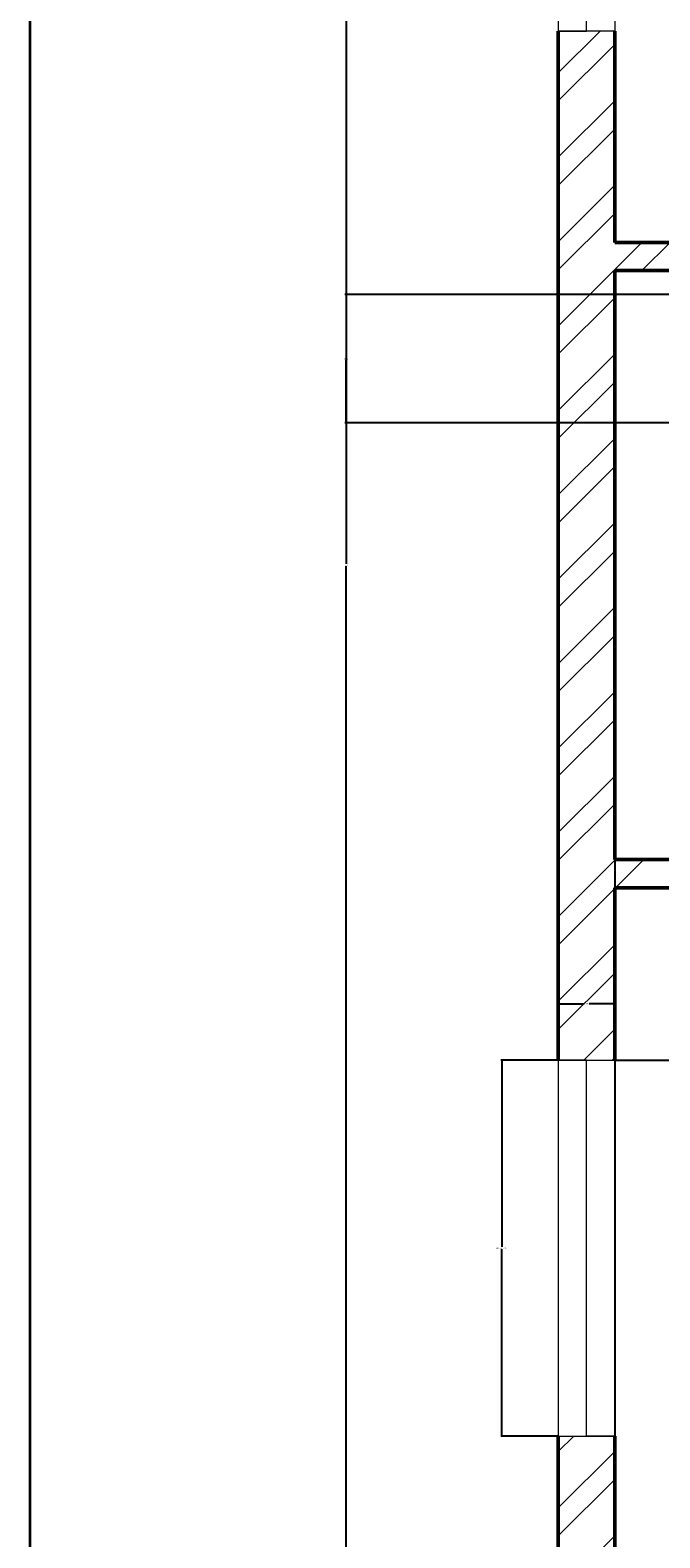
# Model space of a CAD drawing. Units: inches. Extents: x 2310 to 2937, y 1113 to 2410.
# Tile 3 of 23: x 2310 to 2411, y 1891 to 2132. Entities that reach past the tile are written whole.
import ezdxf

# ---------------------------------------------------------------- set-up
doc = ezdxf.new("R2010")
doc.units = ezdxf.units.IN
for name, color, linetype, lineweight in [('A-ANNO-DIMS', 2, 'Continuous', 18), ('A-ANNO-TTLB', 7, 'Continuous', 35), ('A-GLAZ', 191, 'Continuous', 20), ('A-WALL', 7, 'Continuous', 50), ('A-WALL-PATT', 85, 'Continuous', 13)]:
    doc.layers.add(name, color=color, linetype=linetype, lineweight=lineweight)
doc.styles.get("Standard").update_dxf_attribs({"font": 'arial.ttf'})
doc.dimstyles.get("Standard").update_dxf_attribs({"dimtxt": 0.18, "dimasz": 0.18, "dimexe": 0.18, "dimexo": 0.0625, "dimgap": 0.09, "dimtad": 0, "dimtih": 1, "dimtoh": 1, "dimdec": 4, "dimzin": 0, "dimdsep": 46, "dimtxsty": 'Standard', "dimcen": 0.09, "dimadec": 0, "dimazin": 0, "dimtfac": 1, "dimtdec": 4, "dimtofl": 0, "dimtmove": 0, "dimatfit": 3, "dimfxl": 1, "dimtolj": 1, "dimtzin": 0, "dimarcsym": 0})

# ---------------------------------------------------------------- blocks, each defined once
blk = doc.blocks.new('WIN-60IN')
for p, q in [((4.5, 60), (0, 60)), ((0, 60), (9, 60)), ((0, 60), (0, 0)), ((4.5, 0), (4.5, 60)), ((9, 60), (9, 0)), ((0, 0), (9, 0)), ((9, 0), (4.5, 0))]:
    blk.add_line(p, q)
blk = doc.blocks.new('*D27')
at = {"layer": 'A-ANNO-DIMS', "color": 0, "lineweight": -2, "transparency": 16777216}
for p, q in [((2394.42, 1967.52), (2385.31, 1967.52)), ((2385.49, 1967.34), (2385.49, 1937.71)), ((2385.49, 1907.7), (2385.49, 1937.34)), ((2394.42, 1907.52), (2385.31, 1907.52))]:
    blk.add_line(p, q, dxfattribs=at)
at = {"layer": 'A-ANNO-DIMS', "color": 0, "transparency": 16777216}
for points in [[(2385.46, 1967.34), (2385.52, 1967.34), (2385.49, 1967.52)], [(2385.46, 1907.7), (2385.52, 1907.7), (2385.49, 1907.52)]]:
    blk.add_solid(points, dxfattribs=at)
at = {"layer": 'Defpoints', "color": 0, "transparency": 16777216}
for p in [(2385.49, 1967.52), (2394.49, 1967.52), (2394.49, 1907.52)]:
    blk.add_point(p, dxfattribs=at)
at = {"layer": 'A-ANNO-DIMS', "color": 0, "transparency": 16777216, "insert": (2385.49, 1937.52), "char_height": 0.18, "attachment_point": 5}
blk.add_mtext('\\A1;WINDOW 60 TYP.', dxfattribs=at)
blk = doc.blocks.new('*D28')
at = {"layer": 'A-ANNO-DIMS', "color": 0, "lineweight": -2, "transparency": 16777216}
for p, q in [((2394.49, 1967.58), (2394.49, 1976.7)), ((2394.67, 1976.52), (2398.53, 1976.52)), ((2403.31, 1976.52), (2399.44, 1976.52)), ((2403.49, 1967.58), (2403.49, 1976.7))]:
    blk.add_line(p, q, dxfattribs=at)
at = {"layer": 'A-ANNO-DIMS', "color": 0, "transparency": 16777216}
for points in [[(2394.67, 1976.55), (2394.67, 1976.49), (2394.49, 1976.52)], [(2403.31, 1976.55), (2403.31, 1976.49), (2403.49, 1976.52)]]:
    blk.add_solid(points, dxfattribs=at)
at = {"layer": 'Defpoints', "color": 0, "transparency": 16777216}
for p in [(2403.49, 1976.52), (2394.49, 1967.52), (2403.49, 1967.52)]:
    blk.add_point(p, dxfattribs=at)
at = {"layer": 'A-ANNO-DIMS', "color": 0, "transparency": 16777216, "insert": (2398.99, 1976.52), "char_height": 0.18, "attachment_point": 5}
blk.add_mtext('\\A1;9 TYP.', dxfattribs=at)
blk = doc.blocks.new('*D40')
at = {"layer": 'A-ANNO-DIMS', "color": 0, "lineweight": -2, "transparency": 16777216}
for p, q in [((2394.42, 2356.51), (2360.46, 2356.51)), ((2360.64, 2356.33), (2360.64, 2046.7)), ((2360.64, 1736.69), (2360.64, 2046.33)), ((2394.42, 1736.51), (2360.46, 1736.51))]:
    blk.add_line(p, q, dxfattribs=at)
at = {"layer": 'A-ANNO-DIMS', "color": 0, "transparency": 16777216}
for points in [[(2360.61, 2356.33), (2360.67, 2356.33), (2360.64, 2356.51)], [(2360.61, 1736.69), (2360.67, 1736.69), (2360.64, 1736.51)]]:
    blk.add_solid(points, dxfattribs=at)
at = {"layer": 'Defpoints', "color": 0, "transparency": 16777216}
for p in [(2360.64, 2356.51), (2394.49, 2356.51), (2394.49, 1736.51)]:
    blk.add_point(p, dxfattribs=at)
at = {"layer": 'A-ANNO-DIMS', "color": 0, "transparency": 16777216, "insert": (2360.64, 2046.51), "char_height": 0.18, "attachment_point": 5}
blk.add_mtext('\\A1;620', dxfattribs=at)
blk = doc.blocks.new('*D57')
at = {"layer": 'A-ANNO-DIMS', "color": 0, "lineweight": -2, "transparency": 16777216}
for p, q in [((2403.55, 1995.01), (2858.02, 1995.01)), ((2857.84, 1994.83), (2857.84, 1981.45)), ((2857.84, 1967.7), (2857.84, 1981.09)), ((2403.55, 1967.52), (2858.02, 1967.52))]:
    blk.add_line(p, q, dxfattribs=at)
at = {"layer": 'A-ANNO-DIMS', "color": 0, "transparency": 16777216}
for points in [[(2857.81, 1994.83), (2857.87, 1994.83), (2857.84, 1995.01)], [(2857.81, 1967.7), (2857.87, 1967.7), (2857.84, 1967.52)]]:
    blk.add_solid(points, dxfattribs=at)
at = {"layer": 'Defpoints', "color": 0, "transparency": 16777216}
for p in [(2403.49, 1995.01), (2403.49, 1967.52), (2857.84, 1967.52)]:
    blk.add_point(p, dxfattribs=at)
at = {"layer": 'A-ANNO-DIMS', "color": 0, "transparency": 16777216, "insert": (2857.84, 1981.27), "char_height": 0.18, "attachment_point": 5}
blk.add_mtext('\\A1;27.49', dxfattribs=at)
blk = doc.blocks.new('*D65')
at = {"layer": 'A-ANNO-DIMS', "color": 0, "lineweight": -2, "transparency": 16777216}
for p, q in [((2403.49, 2093.45), (2403.49, 1649.5)), ((2436.46, 2093.45), (2436.46, 1649.5)), ((2403.67, 1649.68), (2419.58, 1649.68)), ((2436.28, 1649.68), (2420.37, 1649.68))]:
    blk.add_line(p, q, dxfattribs=at)
at = {"layer": 'A-ANNO-DIMS', "color": 0, "transparency": 16777216}
for points in [[(2403.67, 1649.71), (2403.67, 1649.65), (2403.49, 1649.68)], [(2436.28, 1649.71), (2436.28, 1649.65), (2436.46, 1649.68)]]:
    blk.add_solid(points, dxfattribs=at)
at = {"layer": 'Defpoints', "color": 0, "transparency": 16777216}
for p in [(2403.49, 2093.51), (2436.46, 2093.51), (2436.46, 1649.68)]:
    blk.add_point(p, dxfattribs=at)
at = {"layer": 'A-ANNO-DIMS', "color": 0, "transparency": 16777216, "insert": (2419.98, 1649.68), "char_height": 0.18, "attachment_point": 5}
blk.add_mtext('\\A1;32.98', dxfattribs=at)
blk = doc.blocks.new('*D67')
at = {"layer": 'A-ANNO-DIMS', "color": 0, "lineweight": -2, "transparency": 16777216}
for p, q in [((2684.42, 2089.69), (2360.46, 2089.69)), ((2360.64, 2089.51), (2360.64, 2079.64)), ((2360.64, 2069.41), (2360.64, 2079.28)), ((2684.42, 2069.23), (2360.46, 2069.23))]:
    blk.add_line(p, q, dxfattribs=at)
at = {"layer": 'A-ANNO-DIMS', "color": 0, "transparency": 16777216}
for points in [[(2360.61, 2089.51), (2360.67, 2089.51), (2360.64, 2089.69)], [(2360.61, 2069.41), (2360.67, 2069.41), (2360.64, 2069.23)]]:
    blk.add_solid(points, dxfattribs=at)
at = {"layer": 'Defpoints', "color": 0, "transparency": 16777216}
for p in [(2360.64, 2089.69), (2684.49, 2089.69), (2684.49, 2069.23)]:
    blk.add_point(p, dxfattribs=at)
at = {"layer": 'A-ANNO-DIMS', "color": 0, "transparency": 16777216, "insert": (2360.64, 2079.46), "char_height": 0.18, "attachment_point": 5}
blk.add_mtext('\\A1;20.46', dxfattribs=at)

msp = doc.modelspace()

# ---------------------------------------------------------------- hatches: boundary and pattern name
at = {"layer": 'A-WALL-PATT'}
h = msp.add_hatch(dxfattribs=at)
h.set_pattern_fill('ANSI32', color=256)
h.paths.add_polyline_path([(2639.1394, 2356.5139), (2563.662, 2356.5139), (2563.662, 2347.5139), (2606.9859, 2347.5139), (2606.9859, 2210.5139), (2514.2692, 2210.5139), (2514.2692, 2206.0139), (2606.9859, 2206.0139), (2606.9859, 2098.0139), (2602.689, 2098.0139), (2602.689, 2093.5139), (2615.5262, 2093.5139), (2615.5262, 2095.7639), (2615.5262, 2098.0139), (2611.4859, 2098.0139), (2611.4859, 2206.0139), (2703.9391, 2206.0139), (2703.9391, 2208.2639), (2703.9391, 2210.5139), (2611.4859, 2210.5139), (2611.4859, 2347.5139), (2639.1394, 2347.5139)])
h.paths.add_polyline_path([(2823.9859, 2356.5139), (2699.1394, 2356.5139), (2699.1394, 2347.5139), (2738.4859, 2347.5139), (2738.4859, 2343.9266), (2742.9859, 2343.9266), (2742.9859, 2347.5139), (2814.9859, 2347.5139), (2814.9859, 2336.76), (2823.9859, 2336.76)])
h.paths.add_polyline_path([(2823.9859, 2312.76), (2814.9859, 2312.76), (2814.9859, 2299.5139), (2742.9859, 2299.5139), (2742.9859, 2323.0159), (2740.7359, 2323.0159), (2738.4859, 2323.0159), (2738.4859, 2210.5139), (2734.5483, 2210.5139), (2734.5483, 2206.0139), (2746.8769, 2206.0139), (2746.8769, 2208.2639), (2746.8769, 2210.5139), (2742.9859, 2210.5139), (2742.9859, 2295.0139), (2814.9859, 2295.0139), (2814.9859, 2269.8977), (2823.9859, 2269.8977)])
h.paths.add_polyline_path([(2823.9859, 2210.5139), (2823.9859, 2233.8977), (2819.4859, 2233.8977), (2814.9859, 2233.8977), (2814.9859, 2210.5139), (2769.9745, 2210.5139), (2769.9745, 2206.0139), (2814.9859, 2206.0139), (2814.9859, 2178.3027), (2823.9859, 2178.3027)])
h.paths.add_polyline_path([(2823.9859, 2118.3027), (2819.4859, 2118.3027), (2814.9859, 2118.3027), (2814.9859, 2098.0139), (2647.0333, 2098.0139), (2647.0333, 2093.5139), (2814.9859, 2093.5139), (2814.9859, 1999.5139), (2650.6052, 1999.5139), (2650.6052, 1995.0139), (2814.9859, 1995.0139), (2814.9859, 1969.9784), (2823.9859, 1969.9784)])
h.paths.add_polyline_path([(2403.4859, 2093.5139), (2569.9888, 2093.5139), (2569.9888, 2095.7639), (2569.9888, 2098.0139), (2403.4859, 2098.0139), (2403.4859, 2131.7587), (2394.4859, 2131.7587), (2394.4859, 1967.522), (2403.4859, 1967.522), (2403.4859, 1995.0139), (2569.8903, 1995.0139), (2569.8903, 1997.2639), (2569.8903, 1999.5139), (2403.4859, 1999.5139)])
h.paths.add_polyline_path([(2503.662, 2356.5139), (2394.4859, 2356.5139), (2394.4859, 2337.9231), (2398.9859, 2337.9231), (2403.4859, 2337.9231), (2403.4859, 2347.5139), (2475.4859, 2347.5139), (2475.4859, 2343.0384), (2479.9859, 2343.0384), (2479.9859, 2347.5139), (2503.662, 2347.5139)])
h.paths.add_polyline_path([(2498.3065, 1745.5139), (2479.9859, 1745.5139), (2479.9859, 1749.1663), (2477.7359, 1749.1663), (2475.4859, 1749.1663), (2475.4859, 1745.5139), (2403.4859, 1745.5139), (2403.4859, 1753.6409), (2398.9859, 1753.6409), (2394.4859, 1753.6409), (2394.4859, 1736.5139), (2498.3065, 1736.5139), (2498.3065, 1741.0139)])
h.paths.add_polyline_path([(2479.9859, 1882.5139), (2483.9367, 1882.5139), (2483.9367, 1887.0139), (2471.5501, 1887.0139), (2471.5501, 1885.1969), (2471.5501, 1882.5139), (2475.4859, 1882.5139), (2475.4859, 1798.0139), (2403.4859, 1798.0139), (2403.4859, 1828.0433), (2402.2852, 1828.0433), (2394.4859, 1828.0433), (2394.4859, 1777.6409), (2403.4859, 1777.6409), (2403.4859, 1793.5139), (2475.4859, 1793.5139), (2475.4859, 1769.1696), (2479.9859, 1769.1696)])
h.paths.add_polyline_path([(2403.4859, 1907.522), (2398.9859, 1907.522), (2394.4859, 1907.522), (2394.4859, 1864.0433), (2403.4859, 1864.0433), (2403.4859, 1882.5139), (2448.9325, 1882.5139), (2448.9325, 1884.7639), (2448.9325, 1887.0139), (2403.4859, 1887.0139)])
h.paths.add_polyline_path([(2702.2061, 1887.0139), (2611.4859, 1887.0139), (2611.4859, 1995.0139), (2615.6132, 1995.0139), (2615.6132, 1999.5139), (2602.4798, 1999.5139), (2602.4798, 1997.2639), (2602.4798, 1995.0139), (2606.9859, 1995.0139), (2606.9859, 1887.0139), (2516.2443, 1887.0139), (2516.2443, 1884.7639), (2516.2443, 1882.5139), (2606.9859, 1882.5139), (2606.9859, 1745.5139), (2558.3065, 1745.5139), (2558.3065, 1736.5139), (2638.8921, 1736.5139), (2638.8921, 1741.0139), (2638.8921, 1745.5139), (2611.4859, 1745.5139), (2611.4859, 1882.5139), (2702.2061, 1882.5139)])
h.paths.add_polyline_path([(2823.9859, 1909.9784), (2819.4859, 1909.9784), (2814.9859, 1909.9784), (2814.9859, 1887.0139), (2769.144, 1887.0139), (2769.144, 1884.7639), (2769.144, 1882.5139), (2814.9859, 1882.5139), (2814.9859, 1854.1704), (2823.9859, 1854.1704)])
h.paths.add_polyline_path([(2823.9859, 1818.1704), (2819.4859, 1818.1704), (2814.9859, 1818.1704), (2814.9859, 1798.0139), (2742.9859, 1798.0139), (2742.9859, 1882.5139), (2746.805, 1882.5139), (2746.805, 1887.0139), (2733.7334, 1887.0139), (2733.7334, 1884.7639), (2733.7334, 1882.5139), (2738.4859, 1882.5139), (2738.4859, 1771.1728), (2740.7359, 1771.1728), (2742.9859, 1771.1728), (2742.9859, 1793.5139), (2814.9859, 1793.5139), (2814.9859, 1783.6684), (2823.9859, 1783.6684)])
h.paths.add_polyline_path([(2823.9859, 1759.6684), (2814.9859, 1759.6684), (2814.9859, 1745.5139), (2742.9859, 1745.5139), (2742.9859, 1748.9831), (2740.7359, 1748.9831), (2738.4859, 1748.9831), (2738.4859, 1745.5139), (2698.8921, 1745.5139), (2698.8921, 1736.5139), (2823.9859, 1736.5139)])

# ---------------------------------------------------------------- linework, layer by layer
at = {"layer": 'A-ANNO-TTLB'}
msp.add_lwpolyline([(2310.2498, 2409.8427), (2937.0534, 2409.8427), (2937.0534, 1616.036), (2310.2498, 1616.036)], close=True, dxfattribs=at)
at = {"layer": 'A-WALL'}
for p, q in [((2394.4859, 2131.7587), (2394.4859, 1967.522)), ((2403.4859, 2131.7587), (2403.4859, 2098.0139)), ((2403.4859, 2098.0139), (2571.5658, 2098.0139)), ((2403.4859, 2093.5139), (2569.9888, 2093.5139)), ((2403.4859, 2093.5139), (2403.4859, 1999.5139)), ((2403.4859, 1999.5139), (2569.8903, 1999.5139)), ((2403.4859, 1995.0139), (2571.4589, 1995.0139)), ((2403.4859, 1995.0139), (2403.4859, 1967.522)), ((2394.4859, 1907.522), (2394.4859, 1864.0433)), ((2403.4859, 1907.522), (2403.4859, 1887.0139))]:
    msp.add_line(p, q, dxfattribs=at)

# ---------------------------------------------------------------- block references
at = {"layer": 'A-GLAZ', "extrusion": (0, 0, -1), "zscale": -1}
msp.add_blockref('WIN-60IN', (-2403.4859, 2131.7587), dxfattribs=at)
at = {"layer": 'A-GLAZ'}
msp.add_blockref('WIN-60IN', (2394.4859, 1907.522), dxfattribs=at)

# ---------------------------------------------------------------- dimensions: what is measured, and where the dimension line sits
at = {"layer": 'A-ANNO-DIMS'}
for base, p1, p2, override, picture, middle in [((2360.6359, 2356.5139), (2394.4859, 1736.5139), (2394.4859, 2356.5139), {"dimdec": 0, "dimlfac": 1, "dimrnd": 0, "dimzin": 0, "dimdsep": 46, "dimlunit": 2}, '*D40', (2360.6359, 2046.5139)), ((2360.6359, 2089.6861), (2684.4859, 2069.228), (2684.4859, 2089.6861), {"dimdec": 2, "dimlfac": 1, "dimrnd": 0, "dimzin": 0, "dimdsep": 46, "dimlunit": 2}, '*D67', (2360.6359, 2079.457)), ((2857.8359, 1967.522), (2403.4859, 1995.0139), (2403.4859, 1967.522), {"dimdec": 2, "dimlfac": 1, "dimrnd": 0, "dimzin": 0, "dimdsep": 46, "dimlunit": 2}, '*D57', (2857.8359, 1981.268))]:
    dim = msp.add_linear_dim(base=base, p1=p1, p2=p2, angle=90, dimstyle='Standard', override=override, dxfattribs=at)
    dim.commit()
    dim.dimension.update_dxf_attribs({"geometry": picture, "text_midpoint": middle})
dim = msp.add_linear_dim(base=(2436.4647, 1649.6807), p1=(2403.4859, 2093.5139), p2=(2436.4647, 2093.5139), dimstyle='Standard', override={"dimdec": 2, "dimlfac": 1, "dimrnd": 0, "dimzin": 0, "dimdsep": 46, "dimlunit": 2}, dxfattribs=at)
dim.commit()
dim.dimension.update_dxf_attribs({"geometry": '*D65', "text_midpoint": (2419.9753, 1649.6807)})
dim = msp.add_linear_dim(base=(2403.4859, 1976.522), p1=(2394.4859, 1967.522), p2=(2403.4859, 1967.522), text='<> TYP.', dimstyle='Standard', override={"dimdec": 0, "dimlfac": 1, "dimrnd": 0, "dimzin": 0, "dimdsep": 46, "dimlunit": 2}, dxfattribs=at)
dim.commit()
dim.dimension.update_dxf_attribs({"geometry": '*D28', "text_midpoint": (2398.9859, 1976.522)})
dim = msp.add_linear_dim(base=(2385.4859, 1967.522), p1=(2394.4859, 1907.522), p2=(2394.4859, 1967.522), angle=90, text='WINDOW <> TYP.', dimstyle='Standard', override={"dimdec": 0, "dimlfac": 1, "dimrnd": 0, "dimzin": 0, "dimdsep": 46, "dimlunit": 2}, dxfattribs=at)
dim.commit()
dim.dimension.update_dxf_attribs({"geometry": '*D27', "text_midpoint": (2385.4859, 1937.522)})

doc.saveas('drawing.dxf')
